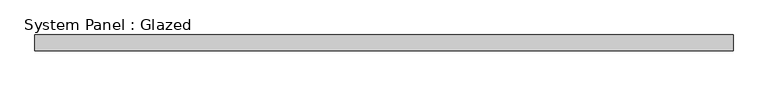
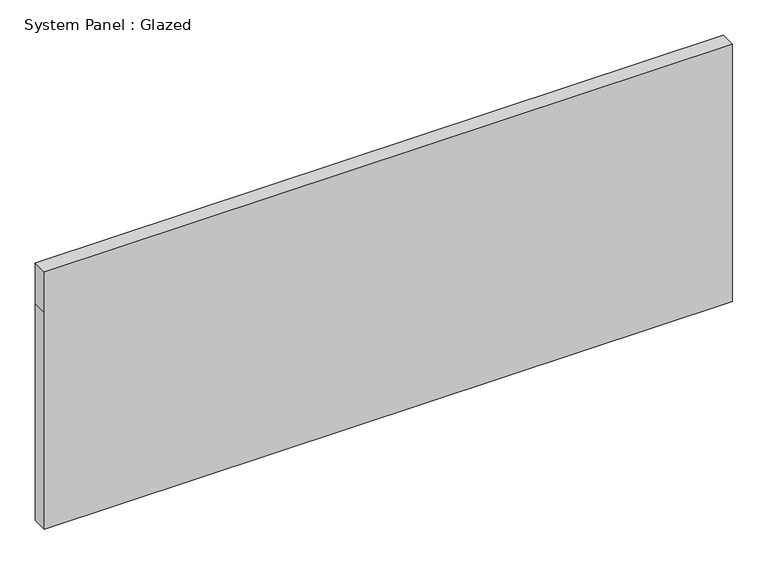
"""IFC4 building model written with IfcOpenShell, lengths in millimetres: plate geometry, System Panel : Glazed."""

from ifc_helpers import new_model, si_unit, frame, origin, place, context, project, spatial, polyline, outline, extrude, source, transform, mapped, element, save


def system_panel_glazed_162183a4(model_context):
    return source(origin(), model_context, "Body", "SweptSolid", [
        extrude(outline(polyline([(0.0, -561.975), (0.0, 561.975), (374.65, 561.975), (444.5, 561.975), (444.5, -561.975), (374.65, -561.975), (0.0, -561.975)])), frame((0.0, -44.45, 0.0), z_axis=(0.0, 1.0, 0.0), x_axis=(0.0, 0.0, 1.0)), (0.0, 0.0, 1.0), 25.4),
    ])


if __name__ == "__main__":
    model = new_model("IFC4")
    model_context = context("Model", 3, world=origin())
    ifc_project = project(units=[si_unit("LENGTHUNIT", "METRE", prefix="MILLI")], contexts=[model_context])
    site = spatial("IfcSite", under=ifc_project)
    building = spatial("IfcBuilding", under=site)
    placement = place(None, origin())
    system_panel_glazed_shape = system_panel_glazed_162183a4(model_context)
    element("IfcPlate", 1, ObjectType="System Panel : Glazed", at=placement, inside=building, context=model_context, shape_type="MappedRepresentation", body=[
        mapped(system_panel_glazed_shape, transform((0.0, 0.0, 0.0), x_axis=(1.0, 0.0, 0.0), y_axis=(0.0, 1.0, 0.0), z_axis=(0.0, 0.0, 1.0))),
    ])
    save(model, "model.ifc")

# Revit data of these elements
# Type "System Panel : Glazed"
#   Construction Type Id = "GSP4R"
#   Analytic Construction = "1/8 in Pilkington single glazing"
#   Visual Light Transmittance = 0.9
#   Solar Heat Gain Coefficient = 0.86
#   Heat Transfer Coefficient (U) = 1.18115 BTU/(h·ft²·°F)
#   Define Thermal Properties by = 1
# Element 1 (IfcPlate, "System Panel : Glazed")
#   Materials on its faces: "GARAGE PANEL"
# Materials
#   "GARAGE PANEL": class "Generic", colour RGB 120 120 120, transparency 0, Cost = 0
